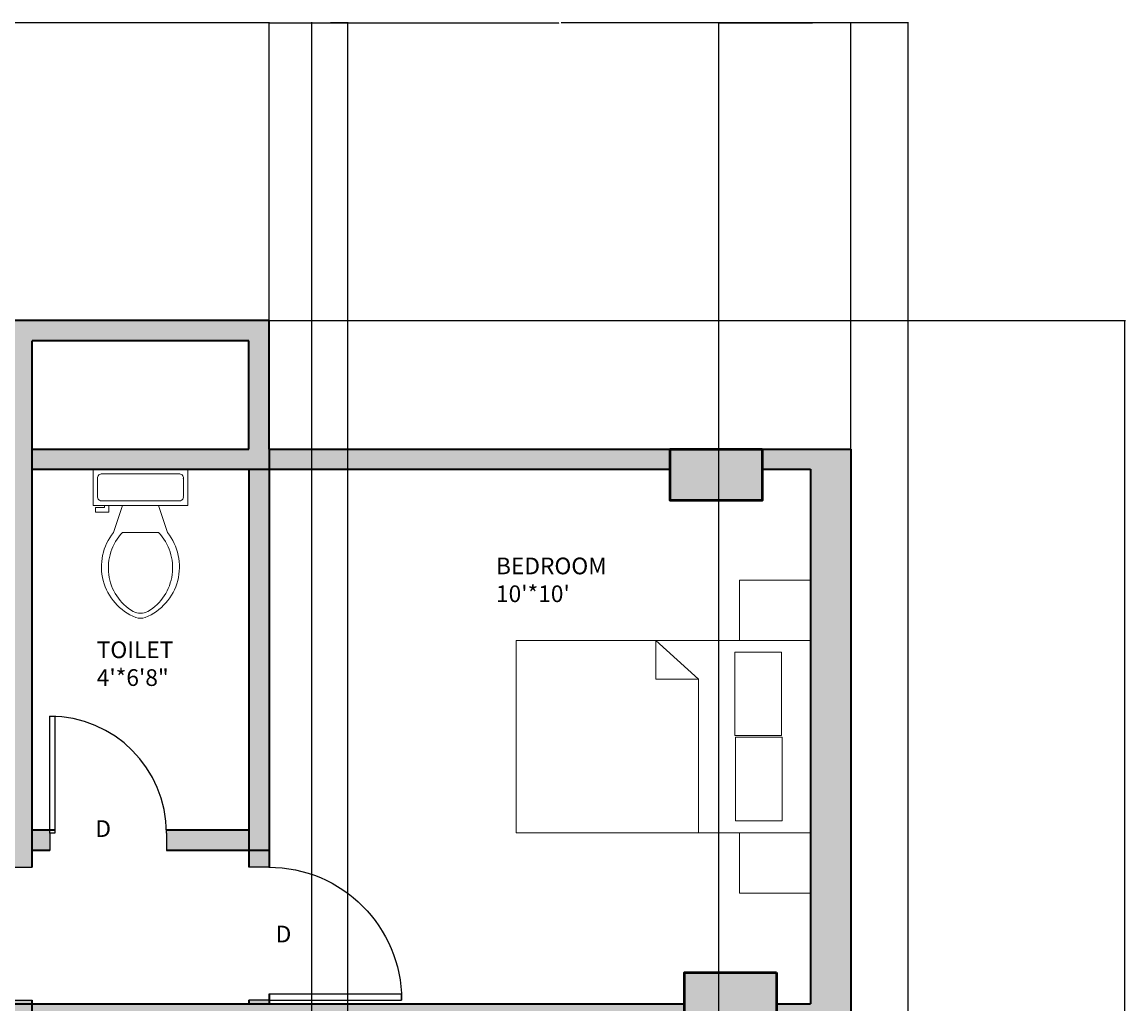
# Model space of a CAD drawing. Units: inches. Extents: x 1998 to 2588, y 1139 to 1977.
# Tile 134 of 134: x 2344 to 2588, y 1760 to 1977. Entities that reach past the tile are written whole.
import ezdxf

# ---------------------------------------------------------------- set-up
doc = ezdxf.new("R2010")
doc.units = ezdxf.units.IN
for name, color, linetype, lineweight in [('A-ANNO-DIMS', 2, 'Continuous', 18), ('A-AREA-IDEN', 7, 'Continuous', 18), ('A-COLS-PATT', 250, 'Continuous', 13), ('A-DOOR-IDEN', 7, 'Continuous', 18), ('A-FLOR-FIXT', 9, 'Continuous', 18), ('A-WALL-PATT', 252, 'Continuous', 13), ('COLUMN', 10, 'Continuous', 50), ('DOOR', 52, 'Continuous', 25), ('FUR', 21, 'Continuous', 18), ('WALL', 200, 'Continuous', 35)]:
    doc.layers.add(name, color=color, linetype=linetype, lineweight=lineweight)
doc.styles.get("Standard").update_dxf_attribs({"font": 'arial.ttf'})
doc.dimstyles.get("Standard").update_dxf_attribs({"dimtxt": 0.18, "dimasz": 0.18, "dimexe": 0.18, "dimexo": 0.0625, "dimgap": 0.09, "dimtad": 0, "dimtih": 1, "dimtoh": 1, "dimdec": 4, "dimzin": 0, "dimdsep": 46, "dimtxsty": 'Standard', "dimcen": 0.09, "dimadec": 0, "dimazin": 0, "dimtfac": 1, "dimtdec": 4, "dimtofl": 0, "dimtmove": 0, "dimatfit": 3, "dimfxl": 1, "dimtolj": 1, "dimtzin": 0, "dimarcsym": 0})

# ---------------------------------------------------------------- blocks, each defined once
blk = doc.blocks.new('*U2')
for p, q in [((0, 0), (0, -6)), ((40, 0), (40, -6))]:
    blk.add_line(p, q)
blk.add_lwpolyline([(0, 0), (0, 40), (1.75, 40), (1.75, 0)], close=True)
blk.add_arc((0, 0), 40, 0, 90)
blk = doc.blocks.new('*U4')
for p, q in [((9.5, -6), (9.5, -2)), ((-10, -8.5), (-8, -8.5)), ((-10, -9.5), (-10, -8.5)), ((-7, -9.5), (-10, -9.5)), ((-8, -8.5), (-8, -8)), ((-7, -8), (-7, -9.5)), ((-4, -8), (-6, -14)), ((4, -8), (6, -14)), ((4, -14), (-4, -14))]:
    blk.add_line(p, q)
blk.add_lwpolyline([(10.5, -8), (10.5, 0), (-10.5, 0), (-10.5, -8)], close=True)
for points in [[(-9.5, -2), (-9.5, -6)], [(8.5, -1), (-8.5, -1)], [(-8.5, -7), (8.5, -7)]]:
    blk.add_lwpolyline(points)
for centre, radius, start, end in [((-8.62, -1.88), 0.884, 81.8699, 188.1301), ((8.62, -1.88), 0.884, 351.8699, 98.1301), ((-8.62, -6.12), 0.884, 171.8699, 278.1301), ((8.62, -6.12), 0.884, 261.8699, 8.1301), ((3.52, -21.58), 12.17, 141.4691, 247.9714), ((4.2, -21.82), 11.33, 136.3677, 238.9468), ((-3.52, -21.58), 12.17, 292.0284, 38.5307), ((-4.2, -21.82), 11.33, 301.053, 43.6321), ((0, -27.88), 4, 245.7318, 294.2682), ((0, -29), 4, 254.8605, 285.1395)]:
    blk.add_arc(centre, radius, start, end)
blk = doc.blocks.new('BED-WITH-NIGHTSTANDS')
for p, q in [((34.22, 56), (24.8, 47.44)), ((34.22, 47.44), (34.22, 56)), ((24.8, 13.42), (24.8, 47.44)), ((24.8, 47.44), (34.22, 47.44))]:
    blk.add_line(p, q)
for points in [[(0, 56), (15.7, 56), (15.7, 69.42), (0, 69.42)], [(0, 56), (65.22, 56), (65.22, 13.42), (0, 13.42)], [(6.37, 34.93), (16.73, 34.93), (16.73, 53.45), (6.37, 53.45)], [(6.25, 16.05), (16.6, 16.05), (16.6, 34.57), (6.25, 34.57)], [(0, 0), (15.7, 0), (15.7, 13.42), (0, 13.42)]]:
    blk.add_lwpolyline(points, close=True)
blk = doc.blocks.new('*D24')
at = {"layer": 'A-ANNO-DIMS', "color": 0, "lineweight": -2, "transparency": 16777216}
for p, q in [((2398.54, 1911.23), (2588.31, 1911.23)), ((2588.13, 1911.05), (2588.13, 1570.16)), ((2588.13, 1228.91), (2588.13, 1569.8)), ((2527.54, 1228.73), (2588.31, 1228.73))]:
    blk.add_line(p, q, dxfattribs=at)
at = {"layer": 'A-ANNO-DIMS', "color": 0, "transparency": 16777216}
for points in [[(2588.1, 1911.05), (2588.16, 1911.05), (2588.13, 1911.23)], [(2588.1, 1228.91), (2588.16, 1228.91), (2588.13, 1228.73)]]:
    blk.add_solid(points, dxfattribs=at)
at = {"layer": 'Defpoints', "color": 0, "transparency": 16777216}
for p in [(2398.47, 1911.23), (2588.13, 1911.23), (2527.47, 1228.73)]:
    blk.add_point(p, dxfattribs=at)
at = {"layer": 'A-ANNO-DIMS', "color": 0, "transparency": 16777216, "insert": (2588.13, 1569.98), "char_height": 0.18, "attachment_point": 5}
blk.add_mtext('\\A1;682.5', dxfattribs=at)
blk = doc.blocks.new('*D26')
at = {"layer": 'A-ANNO-DIMS', "color": 0, "lineweight": -2, "transparency": 16777216}
for p, q in [((2222.97, 1911.29), (2222.97, 1977.36)), ((2398.47, 1911.29), (2398.47, 1977.36)), ((2223.15, 1977.18), (2310.34, 1977.18)), ((2398.29, 1977.18), (2311.11, 1977.18))]:
    blk.add_line(p, q, dxfattribs=at)
at = {"layer": 'A-ANNO-DIMS', "color": 0, "transparency": 16777216}
for points in [[(2223.15, 1977.21), (2223.15, 1977.15), (2222.97, 1977.18)], [(2398.29, 1977.21), (2398.29, 1977.15), (2398.47, 1977.18)]]:
    blk.add_solid(points, dxfattribs=at)
at = {"layer": 'Defpoints', "color": 0, "transparency": 16777216}
for p in [(2398.47, 1977.18), (2222.97, 1911.23), (2398.47, 1911.23)]:
    blk.add_point(p, dxfattribs=at)
at = {"layer": 'A-ANNO-DIMS', "color": 0, "transparency": 16777216, "insert": (2310.72, 1977.18), "char_height": 0.18, "attachment_point": 5}
blk.add_mtext('\\A1;175.5', dxfattribs=at)
blk = doc.blocks.new('*D27')
at = {"layer": 'A-ANNO-DIMS', "color": 0, "lineweight": -2, "transparency": 16777216}
for p, q in [((2398.47, 1882.79), (2398.47, 1977.36)), ((2527.47, 1882.79), (2527.47, 1977.36)), ((2398.65, 1977.18), (2462.69, 1977.18)), ((2527.29, 1977.18), (2463.25, 1977.18))]:
    blk.add_line(p, q, dxfattribs=at)
at = {"layer": 'A-ANNO-DIMS', "color": 0, "transparency": 16777216}
for points in [[(2398.65, 1977.21), (2398.65, 1977.15), (2398.47, 1977.18)], [(2527.29, 1977.21), (2527.29, 1977.15), (2527.47, 1977.18)]]:
    blk.add_solid(points, dxfattribs=at)
at = {"layer": 'Defpoints', "color": 0, "transparency": 16777216}
for p in [(2527.47, 1977.18), (2398.47, 1882.73), (2527.47, 1882.73)]:
    blk.add_point(p, dxfattribs=at)
at = {"layer": 'A-ANNO-DIMS', "color": 0, "transparency": 16777216, "insert": (2462.97, 1977.18), "char_height": 0.18, "attachment_point": 5}
blk.add_mtext('\\A1;129', dxfattribs=at)
blk = doc.blocks.new('*D31')
at = {"layer": 'A-ANNO-DIMS', "color": 0, "lineweight": -2, "transparency": 16777216}
for p, q in [((2498.18, 1636.79), (2498.18, 1977.36)), ((2540.18, 1636.79), (2540.18, 1977.36)), ((2498.36, 1977.18), (2518.96, 1977.18)), ((2540, 1977.18), (2519.4, 1977.18))]:
    blk.add_line(p, q, dxfattribs=at)
at = {"layer": 'A-ANNO-DIMS', "color": 0, "transparency": 16777216}
for points in [[(2498.36, 1977.21), (2498.36, 1977.15), (2498.18, 1977.18)], [(2540, 1977.21), (2540, 1977.15), (2540.18, 1977.18)]]:
    blk.add_solid(points, dxfattribs=at)
at = {"layer": 'Defpoints', "color": 0, "transparency": 16777216}
for p in [(2540.18, 1977.18), (2498.18, 1636.73), (2540.18, 1636.73)]:
    blk.add_point(p, dxfattribs=at)
at = {"layer": 'A-ANNO-DIMS', "color": 0, "transparency": 16777216, "insert": (2519.18, 1977.18), "char_height": 0.18, "attachment_point": 5}
blk.add_mtext('\\A1;42', dxfattribs=at)
blk = doc.blocks.new('*D32')
at = {"layer": 'A-ANNO-DIMS', "color": 0, "lineweight": -2, "transparency": 16777216}
for p, q in [((2407.97, 1636.79), (2407.97, 1977.36)), ((2415.97, 1636.79), (2415.97, 1977.36)), ((2408.15, 1977.18), (2411.82, 1977.18)), ((2415.79, 1977.18), (2412.12, 1977.18))]:
    blk.add_line(p, q, dxfattribs=at)
at = {"layer": 'A-ANNO-DIMS', "color": 0, "transparency": 16777216}
for points in [[(2408.15, 1977.21), (2408.15, 1977.15), (2407.97, 1977.18)], [(2415.79, 1977.21), (2415.79, 1977.15), (2415.97, 1977.18)]]:
    blk.add_solid(points, dxfattribs=at)
at = {"layer": 'Defpoints', "color": 0, "transparency": 16777216}
for p in [(2415.97, 1977.18), (2407.97, 1636.73), (2415.97, 1636.73)]:
    blk.add_point(p, dxfattribs=at)
at = {"layer": 'A-ANNO-DIMS', "color": 0, "transparency": 16777216, "insert": (2411.97, 1977.18), "char_height": 0.18, "attachment_point": 5}
blk.add_mtext('\\A1;8', dxfattribs=at)

msp = doc.modelspace()

# ---------------------------------------------------------------- hatches: boundary and pattern name
at = {"layer": 'A-COLS-PATT'}
h = msp.add_hatch(color=256, dxfattribs=at)
h.dxf.hatch_style = 1
h.paths.add_polyline_path([(2099.4125, 1888.7324), (2087.9729, 1888.7324), (2087.9729, 1868.3278), (2099.4125, 1868.3278)])
h.paths.add_polyline_path([(2234.4125, 1888.7324), (2222.9729, 1888.7324), (2222.9729, 1868.3278), (2234.4125, 1868.3278)])
h.paths.add_polyline_path([(2341.4729, 1886.637), (2330.0332, 1886.637), (2330.0332, 1866.2324), (2341.4729, 1866.2324)])
h.paths.add_polyline_path([(2507.8006, 1882.7324), (2487.396, 1882.7324), (2487.396, 1871.2927), (2507.8006, 1871.2927)])
h.paths.add_polyline_path([(2510.9729, 1766.672), (2490.5682, 1766.672), (2490.5682, 1755.2324), (2510.9729, 1755.2324)])
h.paths.add_polyline_path([(2345.9729, 1759.7324), (2334.5332, 1759.7324), (2334.5332, 1739.3278), (2345.9729, 1739.3278)])
h.paths.add_polyline_path([(2234.4125, 1774.3318), (2222.9729, 1774.3318), (2222.9729, 1753.9272), (2234.4125, 1753.9272)])
h.paths.add_polyline_path([(2099.4125, 1775.637), (2087.9729, 1775.637), (2087.9729, 1755.2324), (2099.4125, 1755.2324)])
h.paths.add_polyline_path([(2098.0956, 1593.7241), (2077.691, 1593.7241), (2077.691, 1582.2845), (2098.0956, 1582.2845)])
h.paths.add_polyline_path([(2227.4729, 1604.637), (2216.0332, 1604.637), (2216.0332, 1584.2324), (2227.4729, 1584.2324)])
h.paths.add_polyline_path([(2345.9729, 1647.5211), (2334.5332, 1647.5211), (2334.5332, 1627.1165), (2345.9729, 1627.1165)])
h.paths.add_polyline_path([(2522.3775, 1641.2324), (2501.9729, 1641.2324), (2501.9729, 1629.7927), (2522.3775, 1629.7927)])
h.paths.add_polyline_path([(2522.3775, 1480.7324), (2501.9729, 1480.7324), (2501.9729, 1469.2927), (2522.3775, 1469.2927)])
h.paths.add_polyline_path([(2345.9729, 1488.5616), (2334.5332, 1488.5616), (2334.5332, 1468.1569), (2345.9729, 1468.1569)])
h.paths.add_polyline_path([(2234.4125, 1486.137), (2227.4729, 1486.137), (2227.4729, 1465.7324), (2234.4125, 1465.7324)])
h.paths.add_polyline_path([(2227.4729, 1486.137), (2222.9729, 1486.137), (2222.9729, 1465.7324), (2227.4729, 1465.7324)])
h.paths.add_polyline_path([(2108.3775, 1470.2324), (2087.9729, 1470.2324), (2087.9729, 1458.7927), (2108.3775, 1458.7927)])
h.paths.add_polyline_path([(2096.9729, 1365.5012), (2087.9729, 1365.5012), (2087.9729, 1345.0966), (2096.9729, 1345.0966)])
h.paths.add_polyline_path([(2087.9729, 1365.5012), (2085.5332, 1365.5012), (2085.5332, 1345.0966), (2087.9729, 1345.0966)])
h.paths.add_polyline_path([(2234.4125, 1285.137), (2222.9729, 1285.137), (2222.9729, 1264.7324), (2234.4125, 1264.7324)])
h.paths.add_polyline_path([(2345.9729, 1285.137), (2334.5332, 1285.137), (2334.5332, 1264.7324), (2345.9729, 1264.7324)])
h.paths.add_polyline_path([(2503.1458, 1240.172), (2482.7412, 1240.172), (2482.7412, 1228.7324), (2503.1458, 1228.7324)])
h.paths.add_polyline_path([(2510.9729, 1369.172), (2490.5682, 1369.172), (2490.5682, 1357.7324), (2510.9729, 1357.7324)])
at = {"layer": 'A-WALL-PATT'}
h = msp.add_hatch(color=256, dxfattribs=at)
h.dxf.hatch_style = 1
h.paths.add_polyline_path([(2227.4729, 1911.2324), (2222.9729, 1911.2324), (2222.9729, 1888.7324), (2227.4729, 1888.7324)])
h.paths.add_polyline_path([(2236.4493, 1870.3636), (2236.4493, 1875.2324), (2234.4125, 1875.2324), (2234.4125, 1868.3278), (2227.4729, 1868.3278), (2227.4729, 1866.2324), (2236.4493, 1866.2324)])
h.paths.add_polyline_path([(2330.0332, 1875.2324), (2263.9907, 1875.2324), (2263.9907, 1866.2324), (2330.0332, 1866.2324)])
h.paths.add_polyline_path([(2345.9729, 1906.7324), (2393.9729, 1906.7324), (2393.9729, 1882.7324), (2345.9729, 1882.7324), (2345.9729, 1878.2324), (2393.9729, 1878.2324), (2398.4729, 1878.2324), (2398.4729, 1882.7324), (2398.4729, 1911.2324), (2345.9729, 1911.2324), (2341.4729, 1911.2324), (2341.4729, 1866.2324), (2341.4729, 1790.0412), (2345.9729, 1790.0412), (2345.9729, 1875.2324)])
h.paths.add_polyline_path([(2398.4729, 1878.2324), (2393.9729, 1878.2324), (2393.9729, 1798.2324), (2393.9729, 1793.7324), (2398.4729, 1793.7324)], flags=17)
h.paths.add_polyline_path([(2393.9729, 1798.2324), (2375.7311, 1798.2324, -0.00596797), (2375.7384, 1797.6146), (2375.7384, 1793.7324), (2393.9729, 1793.7324)], flags=17)
h.paths.add_polyline_path([(2349.8569, 1797.6146), (2349.8569, 1798.2324), (2345.9729, 1798.2324), (2345.9729, 1793.7324), (2349.8569, 1793.7324)], flags=17)
h.paths.add_polyline_path([(2398.4729, 1793.7324), (2393.9729, 1793.7324), (2393.9729, 1790.0412), (2398.4729, 1790.0412)], flags=17)
h.paths.add_polyline_path([(2527.4729, 1882.7324), (2507.8006, 1882.7324), (2507.8006, 1878.2324), (2518.4729, 1878.2324), (2518.4729, 1759.7324), (2510.9729, 1759.7324), (2510.9729, 1755.2324), (2527.4729, 1755.2324)])
h.paths.add_polyline_path([(2487.396, 1882.7324), (2398.4729, 1882.7324), (2398.4729, 1878.2324), (2487.396, 1878.2324)])
h.paths.add_polyline_path([(2490.5682, 1759.7324), (2345.9729, 1759.7324), (2345.9729, 1755.2324), (2490.5682, 1755.2324)])
h.paths.add_polyline_path([(2398.4729, 1760.5844), (2398.3914, 1760.5844), (2393.9729, 1760.5844), (2393.9729, 1759.7324), (2398.4729, 1759.7324)])
h.paths.add_polyline_path([(2334.5332, 1759.7324), (2234.4125, 1759.7324), (2234.4125, 1755.2324), (2334.5332, 1755.2324)])
h.paths.add_polyline_path([(2345.9729, 1760.5844), (2341.5543, 1760.5844), (2341.4729, 1760.5844), (2341.4729, 1759.7324), (2345.9729, 1759.7324)])
h.paths.add_polyline_path([(2222.9729, 1759.7324), (2221.7204, 1759.7324), (2221.7204, 1755.2324), (2222.9729, 1755.2324)])
h.paths.add_polyline_path([(2061.4729, 1702.7324), (2059.4729, 1702.7324), (2059.4729, 1584.2324), (2061.4729, 1584.2324)])
h.paths.add_polyline_path([(2061.4729, 1584.2324), (2059.4729, 1584.2324), (2059.4729, 1470.2324), (2061.4729, 1470.2324)])
h.paths.add_polyline_path([(2510.9729, 1469.2927), (2501.9729, 1469.2927), (2501.9729, 1369.172), (2510.9729, 1369.172)])
h.paths.add_polyline_path([(2227.4729, 1369.7324), (2227.4729, 1417.7324), (2221.4126, 1417.7324), (2221.4126, 1413.2324), (2222.9729, 1413.2324), (2222.9729, 1293.2324), (2222.9729, 1285.137), (2227.4729, 1285.137)])

# ---------------------------------------------------------------- linework, layer by layer
at = {"layer": 'COLUMN'}
for points in [[(2507.8006, 1882.7324), (2507.8006, 1871.2927), (2487.396, 1871.2927), (2487.396, 1882.7324)], [(2510.9729, 1766.672), (2510.9729, 1755.2324), (2490.5682, 1755.2324), (2490.5682, 1766.672)]]:
    msp.add_lwpolyline(points, close=True, dxfattribs=at)
at = {"layer": 'WALL'}
for p, q in [((2345.9729, 1911.2324), (2222.9729, 1911.2324)), ((2398.4729, 1911.2324), (2345.9729, 1911.2324)), ((2398.4729, 1882.7324), (2398.4729, 1911.2324)), ((2345.9729, 1875.2324), (2345.9729, 1906.7324)), ((2393.9729, 1906.7324), (2345.9729, 1906.7324)), ((2393.9729, 1882.7324), (2393.9729, 1906.7324)), ((2345.9729, 1882.7324), (2393.9729, 1882.7324)), ((2398.4729, 1882.7324), (2398.4729, 1793.7324)), ((2398.4729, 1882.7324), (2527.4729, 1882.7324)), ((2527.4729, 1882.7324), (2527.4729, 1755.2324)), ((2345.9729, 1878.2324), (2393.9729, 1878.2324)), ((2393.9729, 1878.2324), (2393.9729, 1798.2324)), ((2393.9729, 1878.2324), (2398.4729, 1878.2324)), ((2398.4729, 1878.2324), (2487.396, 1878.2324)), ((2507.8006, 1878.2324), (2518.4729, 1878.2324)), ((2518.4729, 1878.2324), (2518.4729, 1759.7324)), ((2345.9729, 1790.0412), (2345.9729, 1875.2324)), ((2350.9893, 1798.2324), (2345.9729, 1798.2324)), ((2393.9729, 1798.2324), (2375.7311, 1798.2324)), ((2393.9729, 1798.2324), (2393.9729, 1790.0412)), ((2349.8569, 1793.7324), (2345.9729, 1793.7324)), ((2398.4729, 1793.7324), (2375.7384, 1793.7324)), ((2398.4729, 1793.7324), (2398.4729, 1790.041)), ((2341.4729, 1759.7324), (2490.5682, 1759.7324)), ((2345.9729, 1755.2324), (2345.9729, 1760.5844)), ((2393.9729, 1760.5844), (2393.9729, 1759.7324)), ((2398.4729, 1761.8731), (2398.4729, 1759.7324)), ((2510.9729, 1759.7324), (2518.4729, 1759.7324))]:
    msp.add_line(p, q, dxfattribs=at)

# ---------------------------------------------------------------- block references
at = {"layer": 'A-FLOR-FIXT'}
msp.add_blockref('*U4', (2369.9729, 1878.2324), dxfattribs=at)
at = {"layer": 'DOOR', "xscale": 0.647037619250368, "yscale": 0.647037619250368, "zscale": 0.647037619250368}
msp.add_blockref('*U2', (2349.8569, 1797.6146), dxfattribs=at)
at = {"layer": 'DOOR', "yscale": 0.7364194310947476, "zscale": 0.7364194310947476}
for p, xscale, rotation in [((2341.5543, 1760.5844), 0.7364194310947476, 90), ((2398.3914, 1760.5844), -0.7364194310947476, 270)]:
    msp.add_blockref('*U2', p, dxfattribs=dict(at, xscale=xscale, rotation=rotation))
at = {"layer": 'FUR', "extrusion": (0, 0, -1), "zscale": -1}
msp.add_blockref('BED-WITH-NIGHTSTANDS', (-2518.4727, 1784.2703), dxfattribs=at)

# ---------------------------------------------------------------- texts
at = {"layer": 'A-AREA-IDEN', "char_height": 3.69875, "attachment_point": 1}
for s, insert in [("BEDROOM\\P10'*10'", (2448.78, 1858.6624)), ('TOILET\\P4\'*6\'8"', (2360.2758, 1840.0807))]:
    msp.add_mtext_dynamic_manual_height_columns(s, width=110.572713, gutter_width=18.4938, heights=[0], dxfattribs=dict(at, insert=insert))
at = {"layer": 'A-DOOR-IDEN', "char_height": 3.6988, "attachment_point": 1}
for insert in [(2359.9646, 1800.4409), (2399.9376, 1777.0651)]:
    msp.add_mtext_dynamic_manual_height_columns('D', width=110.572713, gutter_width=18.4938, heights=[0], dxfattribs=dict(at, insert=insert))

# ---------------------------------------------------------------- dimensions: what is measured, and where the dimension line sits
at = {"layer": 'A-ANNO-DIMS'}
for base, p1, p2, override, picture, middle in [((2398.4729, 1977.1824), (2222.9729, 1911.2324), (2398.4729, 1911.2324), {"dimdec": 1, "dimlfac": 1, "dimrnd": 0, "dimzin": 0, "dimdsep": 46, "dimlunit": 2}, '*D26', (2310.7229, 1977.1824)), ((2527.4729, 1977.1824), (2398.4729, 1882.7324), (2527.4729, 1882.7324), {"dimdec": 0, "dimlfac": 1, "dimrnd": 0, "dimzin": 0, "dimdsep": 46, "dimlunit": 2}, '*D27', (2462.9729, 1977.1824)), ((2415.9729, 1977.1824), (2407.9729, 1636.7324), (2415.9729, 1636.7324), {"dimdec": 0, "dimlfac": 1, "dimrnd": 0, "dimzin": 0, "dimdsep": 46, "dimlunit": 2}, '*D32', (2411.9729, 1977.1824)), ((2540.1786, 1977.1824), (2498.1786, 1636.7324), (2540.1786, 1636.7324), {"dimdec": 0, "dimlfac": 1, "dimrnd": 0, "dimzin": 0, "dimdsep": 46, "dimlunit": 2}, '*D31', (2519.1786, 1977.1824))]:
    dim = msp.add_linear_dim(base=base, p1=p1, p2=p2, dimstyle='Standard', override=override, dxfattribs=at)
    dim.commit()
    dim.dimension.update_dxf_attribs({"geometry": picture, "text_midpoint": middle})
dim = msp.add_linear_dim(base=(2588.1286, 1911.2324), p1=(2527.4729, 1228.7324), p2=(2398.4729, 1911.2324), angle=90, dimstyle='Standard', override={"dimdec": 1, "dimlfac": 1, "dimrnd": 0, "dimzin": 0, "dimdsep": 46, "dimlunit": 2}, dxfattribs=at)
dim.commit()
dim.dimension.update_dxf_attribs({"geometry": '*D24', "text_midpoint": (2588.1286, 1569.9824)})

doc.saveas('drawing.dxf')
